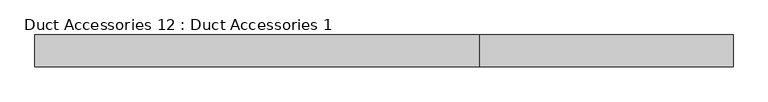
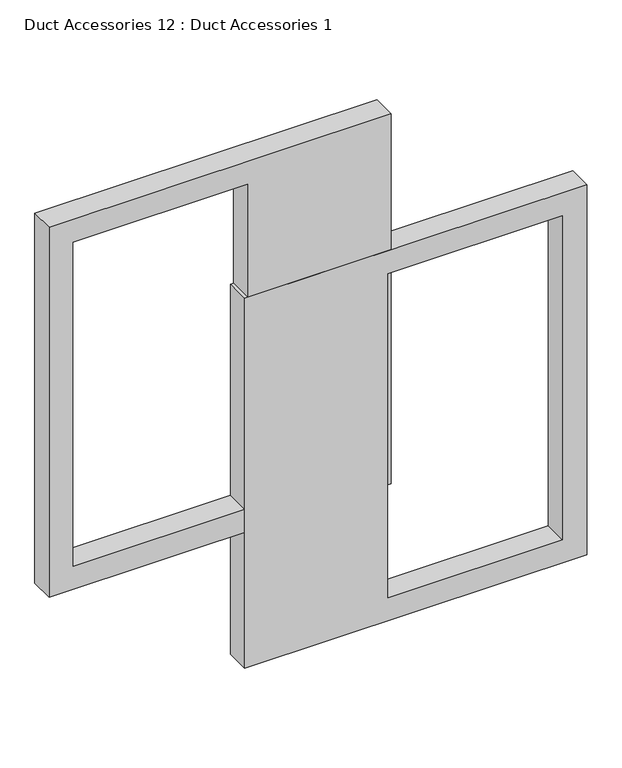
"""IFC4 building model written with IfcOpenShell, lengths in millimetres: damper geometry, Duct Accessories 12 : Duct Accessories 1."""

from ifc_helpers import new_model, si_unit, frame, origin, place, context, project, spatial, polyline, outline, extrude, source, transform, mapped, element, save


def duct_accessories_12_duct_accessories_1_1d6ac5d5(model_context):
    return source(origin(), model_context, "Body", "SweptSolid", [
        extrude(outline(polyline([(4847.1403114, -12928.36893), (3627.9403114, -12928.36893), (3627.9403114, -11861.56893), (4847.1403114, -11861.56893), (4847.1403114, -12928.36893)]), holes=[polyline([(4770.9403114, -12480.9324751), (4770.9403114, -11937.76893), (3704.1403114, -11937.76893), (3704.1403114, -12480.9324751), (4770.9403114, -12480.9324751)])]), frame((0.0, -447.4934478, 0.0), z_axis=(0.0, 1.0, 0.0), x_axis=(0.0, 0.0, 1.0)), (0.0, 0.0, 1.0), 76.2),
        extrude(outline(polyline([(5294.5767663, -12471.5606701), (5294.5767663, -13538.3606701), (4075.3767663, -13538.3606701), (4075.3767663, -12471.5606701), (5294.5767663, -12471.5606701)]), holes=[polyline([(5218.3767663, -12918.997125), (4151.5767663, -12918.997125), (4151.5767663, -13462.1606701), (5218.3767663, -13462.1606701), (5218.3767663, -12918.997125)])]), frame((0.0, -447.4934478, 0.0), z_axis=(0.0, 1.0, 0.0), x_axis=(0.0, 0.0, 1.0)), (0.0, 0.0, 1.0), 76.2),
    ])


if __name__ == "__main__":
    model = new_model("IFC4")
    model_context = context("Model", 3, world=origin())
    ifc_project = project(units=[si_unit("LENGTHUNIT", "METRE", prefix="MILLI")], contexts=[model_context])
    site = spatial("IfcSite", under=ifc_project)
    building = spatial("IfcBuilding", under=site)
    placement = place(None, origin())
    duct_accessories_12_duct_accessories_1_shape = duct_accessories_12_duct_accessories_1_1d6ac5d5(model_context)
    element("IfcDamper", 1, ObjectType="Duct Accessories 12 : Duct Accessories 1", at=placement, inside=building, context=model_context, shape_type="MappedRepresentation", body=[
        mapped(duct_accessories_12_duct_accessories_1_shape, transform((0.0, 0.0, 0.0), x_axis=(1.0, 0.0, 0.0), y_axis=(0.0, 1.0, 0.0), z_axis=(0.0, 0.0, 1.0))),
    ])
    save(model, "model.ifc")

# Revit data of these elements
# Element 1 (IfcDamper, "Duct Accessories 12 : Duct Accessories 1")
#   Materials on its faces: "border"
# Materials
#   "border": class "Generic", colour RGB 144 144 144, transparency 0, Cost = 0
